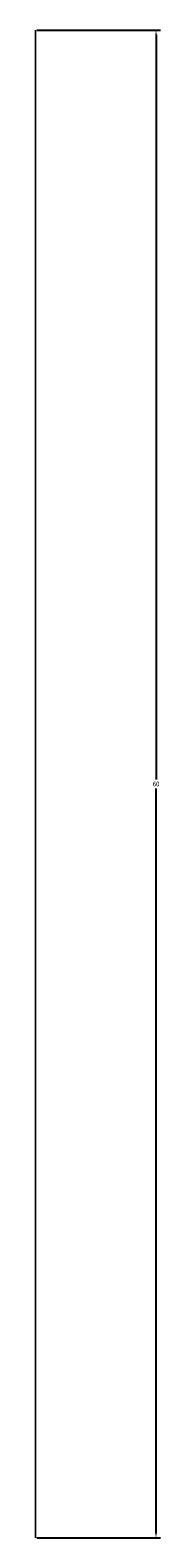
# Model space of a CAD drawing. Units: millimetres. Extents: x 0 to 390, y -312 to 42.
# Tile 1 of 3: x 0 to 5, y -253 to -193. Entities that reach past the tile are written whole.
import ezdxf

# ---------------------------------------------------------------- set-up
doc = ezdxf.new("R2010")
doc.units = ezdxf.units.MM
doc.layers.add('M-CONS', color=8, linetype='Continuous', lineweight=18)
doc.layers.add('M-DIMS', color=2, linetype='Continuous', lineweight=18)
doc.styles.get("Standard").update_dxf_attribs({"font": 'arial.ttf'})
doc.dimstyles.get("Standard").update_dxf_attribs({"dimtxt": 0.18, "dimasz": 0.18, "dimexe": 0.18, "dimexo": 0.0625, "dimgap": 0.09, "dimtad": 0, "dimtih": 1, "dimtoh": 1, "dimdec": 4, "dimzin": 0, "dimdsep": 46, "dimtxsty": 'Standard', "dimcen": 0.09, "dimadec": 0, "dimazin": 0, "dimtfac": 1, "dimtdec": 4, "dimtofl": 0, "dimtmove": 0, "dimatfit": 3, "dimfxl": 1, "dimtolj": 1, "dimtzin": 0, "dimarcsym": 0})

# ---------------------------------------------------------------- blocks, each defined once
blk = doc.blocks.new('*D10')
at = {"layer": 'Defpoints', "color": 0, "transparency": 16777216}
for p in [(0, -193.243), (4.8, -193.243), (0, -253.243)]:
    blk.add_point(p, dxfattribs=at)
at = {"layer": 'M-DIMS', "color": 0, "lineweight": -2, "transparency": 16777216}
for p, q in [((0.062, -193.243), (4.98, -193.243)), ((4.8, -193.423), (4.8, -223.061)), ((4.8, -253.063), (4.8, -223.425)), ((0.062, -253.243), (4.98, -253.243))]:
    blk.add_line(p, q, dxfattribs=at)
at = {"layer": 'M-DIMS', "color": 0, "transparency": 16777216}
for points in [[(4.77, -193.423), (4.83, -193.423), (4.8, -193.243)], [(4.77, -253.063), (4.83, -253.063), (4.8, -253.243)]]:
    blk.add_solid(points, dxfattribs=at)
at = {"layer": 'M-DIMS', "color": 0, "transparency": 16777216, "insert": (4.8, -223.243), "char_height": 0.18, "attachment_point": 5}
blk.add_mtext('\\A1;60', dxfattribs=at)

msp = doc.modelspace()

# ---------------------------------------------------------------- linework, layer by layer
at = {"layer": 'M-CONS', "extrusion": (-1, 0, 0)}
msp.add_lwpolyline([(253.243, 305.854), (253.243, 269.854), (193.243, 269.854), (193.243, 305.854)], close=True, dxfattribs=at)

# ---------------------------------------------------------------- dimensions: what is measured, and where the dimension line sits
at = {"layer": 'M-DIMS'}
dim = msp.add_linear_dim(base=(4.8, -193.243), p1=(0, -253.243), p2=(0, -193.243), angle=90, dimstyle='Standard', override={"dimdec": 0, "dimlfac": 1, "dimrnd": 0, "dimzin": 0, "dimdsep": 46, "dimlunit": 2}, dxfattribs=at)
dim.commit()
dim.dimension.update_dxf_attribs({"geometry": '*D10', "text_midpoint": (4.8, -223.243)})

doc.saveas('drawing.dxf')
